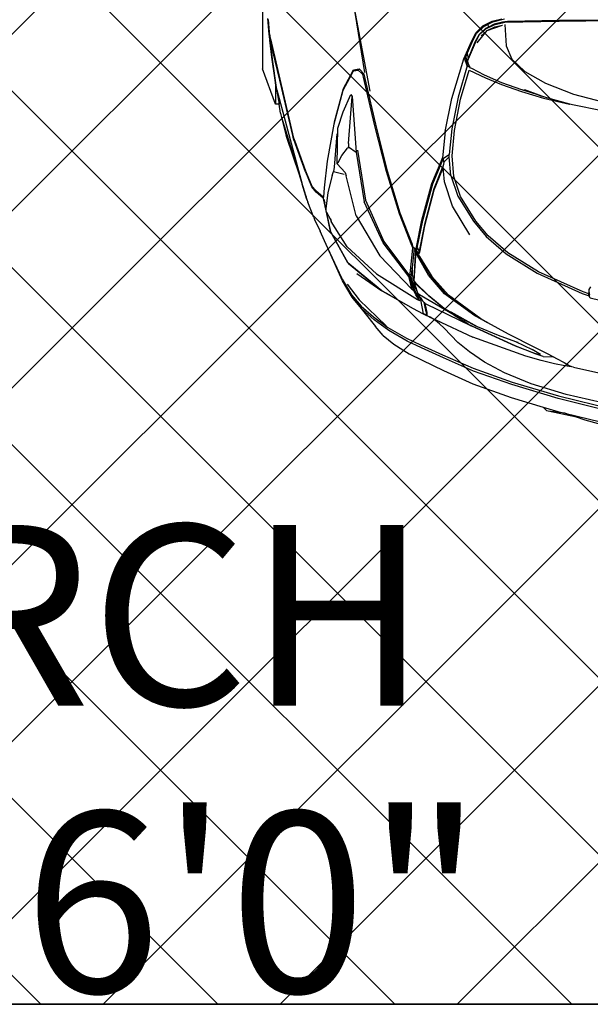
# Model space of a CAD drawing. Units: inches. Extents: x 2167 to 2589, y 1680 to 2489.
# Tile 12 of 38: x 2335 to 2358, y 1688 to 1727. Entities that reach past the tile are written whole.
import ezdxf

# ---------------------------------------------------------------- set-up
doc = ezdxf.new("R2010")
doc.units = ezdxf.units.IN
doc.header["$MEASUREMENT"] = 0
doc.layers.get('0').update_dxf_attribs({"color": 250})
for name, color, linetype, lineweight in [('A-AREA-IDEN', 7, 'Continuous', 18), ('C-PRKG-VEHS', 8, 'Continuous', 13), ('C-PROP', 7, 'Continuous', 35), ('L-PVMT-PATT', 252, 'Continuous', 13)]:
    doc.layers.add(name, color=color, linetype=linetype, lineweight=lineweight)
doc.layers.add('Edges', color=250, linetype='Continuous')
doc.styles.get("Standard").update_dxf_attribs({"font": 'arial.ttf'})

# ---------------------------------------------------------------- blocks, each defined once
blk = doc.blocks.new('Nissan Qashqai pl')
at = {"layer": 'Edges'}
for p, q in [((11.0595, 11.5599), (11.0607, 11.4508)), ((11.0606, 11.5601), (11.0618, 11.4509)), ((11.164, 11.4711), (11.1776, 11.5231)), ((11.6016, 11.5276), (11.5866, 11.4607)), ((11.5884, 11.4499), (11.6076, 11.5276)), ((11.6118, 11.5276), (11.5922, 11.4494)), ((11.6127, 11.4589), (11.6297, 11.5276)), ((11.1877, 11.5111), (11.1791, 11.4696)), ((11.4503, 11.4945), (11.4568, 11.5197)), ((11.5481, 11.471), (11.5571, 11.511)), ((11.435, 11.4947), (11.439, 11.4927)), ((11.439, 11.4927), (11.4437, 11.4925)), ((11.4451, 11.4934), (11.4432, 11.4935)), ((11.4437, 11.4925), (11.4449, 11.4929)), ((11.4445, 11.4833), (11.4478, 11.493)), ((11.4449, 11.4929), (11.4447, 11.4924)), ((11.4449, 11.4929), (11.4461, 11.4934)), ((11.4451, 11.4934), (11.4449, 11.4929)), ((11.4461, 11.4934), (11.4451, 11.4934)), ((11.4479, 11.4933), (11.4461, 11.4934)), ((11.4479, 11.4933), (11.4462, 11.4924)), ((11.4478, 11.493), (11.4462, 11.4924)), ((11.4502, 11.4939), (11.4478, 11.493)), ((11.4503, 11.4945), (11.4479, 11.4932)), ((11.4479, 11.4932), (11.4479, 11.4933)), ((11.4502, 11.4939), (11.4503, 11.4945)), ((11.6277, 11.5063), (11.6224, 11.4874)), ((11.4422, 11.4848), (11.4138, 11.4219)), ((11.4159, 11.42), (11.4445, 11.4833)), ((11.4447, 11.4924), (11.4422, 11.4848)), ((11.4447, 11.4924), (11.4437, 11.4925)), ((11.4462, 11.4924), (11.4447, 11.4924)), ((11.6224, 11.4874), (11.6185, 11.4753)), ((11.1487, 11.4316), (11.164, 11.4711)), ((11.1781, 11.4659), (11.1694, 11.4337)), ((11.1699, 11.4289), (11.178, 11.4652)), ((11.178, 11.4652), (11.1781, 11.4659)), ((11.1791, 11.4696), (11.1781, 11.4659)), ((11.5455, 11.4648), (11.5472, 11.4684)), ((11.5481, 11.471), (11.5467, 11.462)), ((11.6185, 11.4753), (11.6101, 11.4356)), ((11.6174, 11.472), (11.6127, 11.4589)), ((11.6185, 11.4753), (11.6174, 11.472)), ((11.5357, 11.4473), (11.5416, 11.4578)), ((11.5416, 11.4578), (11.5455, 11.4648)), ((11.5461, 11.4587), (11.5434, 11.4445)), ((11.5467, 11.462), (11.5461, 11.4587)), ((11.5866, 11.4607), (11.5715, 11.4115)), ((11.6127, 11.4589), (11.6101, 11.4356)), ((11.6103, 11.4492), (11.6127, 11.4589)), ((11.0607, 11.4508), (11.0621, 11.3784)), ((11.0618, 11.4509), (11.0632, 11.3741)), ((11.5283, 11.4332), (11.5334, 11.4428)), ((11.5326, 11.4397), (11.5333, 11.4423)), ((11.5331, 11.4285), (11.5335, 11.4431)), ((11.5333, 11.4423), (11.5334, 11.4428)), ((11.5334, 11.4428), (11.5335, 11.4431)), ((11.5335, 11.4431), (11.5357, 11.4473)), ((11.5434, 11.4445), (11.5386, 11.4254)), ((11.5691, 11.385), (11.5884, 11.4499)), ((11.5922, 11.4494), (11.5726, 11.3842)), ((11.6042, 11.4286), (11.6103, 11.4492)), ((11.1323, 11.4027), (11.1487, 11.4316)), ((11.1668, 11.4265), (11.1582, 11.4026)), ((11.1605, 11.3977), (11.1699, 11.4289)), ((11.1643, 11.4192), (11.1668, 11.4265)), ((11.1694, 11.4337), (11.1668, 11.4265)), ((11.5202, 11.4171), (11.5283, 11.4332)), ((11.5301, 11.4244), (11.523, 11.4131)), ((11.5331, 11.4285), (11.5292, 11.417)), ((11.5302, 11.4232), (11.5301, 11.4244)), ((11.5386, 11.4254), (11.5325, 11.4038)), ((11.5908, 11.3836), (11.6042, 11.4286)), ((11.6077, 11.4316), (11.6042, 11.4286)), ((11.6094, 11.4335), (11.6077, 11.4316)), ((11.6101, 11.4356), (11.6094, 11.4335)), ((11.1576, 11.3983), (11.1643, 11.4192)), ((11.1577, 11.3977), (11.1643, 11.4192)), ((11.1643, 11.4192), (11.1583, 11.4019)), ((11.4138, 11.4219), (11.3872, 11.3788)), ((11.3888, 11.3764), (11.4159, 11.42)), ((11.5013, 11.3791), (11.5202, 11.4171)), ((11.5118, 11.3894), (11.523, 11.4131)), ((11.5292, 11.417), (11.5179, 11.389)), ((11.5179, 11.389), (11.5285, 11.4163)), ((11.5285, 11.4163), (11.5302, 11.4232)), ((11.5715, 11.4115), (11.5562, 11.3741)), ((11.1148, 11.3843), (11.1323, 11.4027)), ((11.1475, 11.37), (11.1577, 11.3977)), ((11.1505, 11.37), (11.1605, 11.3977)), ((11.5325, 11.4038), (11.5057, 11.3296)), ((11.0962, 11.3766), (11.1148, 11.3843)), ((11.5179, 11.389), (11.488, 11.3234)), ((11.49, 11.3275), (11.5179, 11.389)), ((11.5028, 11.365), (11.5118, 11.3894)), ((11.5118, 11.3894), (11.513, 11.3927)), ((11.5496, 11.33), (11.5691, 11.385)), ((11.5726, 11.3842), (11.5535, 11.3303)), ((11.5716, 11.3297), (11.5908, 11.3836)), ((11.0614, 11.3569), (11.0581, 11.3704)), ((11.0624, 11.3576), (11.0582, 11.3742)), ((11.0621, 11.3784), (11.0622, 11.3745)), ((11.0622, 11.3745), (11.063, 11.3714)), ((11.063, 11.3714), (11.0659, 11.3594)), ((11.0632, 11.3741), (11.0641, 11.3708)), ((11.0641, 11.3708), (11.0669, 11.3592)), ((11.0662, 11.3744), (11.0962, 11.3766)), ((11.0696, 11.3606), (11.0671, 11.3711)), ((11.0747, 11.3498), (11.0671, 11.3711)), ((11.1369, 11.3455), (11.1475, 11.37)), ((11.1412, 11.3473), (11.1505, 11.37)), ((11.3872, 11.3788), (11.3635, 11.3513)), ((11.3645, 11.3484), (11.3888, 11.3764)), ((11.4852, 11.3502), (11.5013, 11.3791)), ((11.5562, 11.3741), (11.541, 11.3459)), ((11.0682, 11.3438), (11.0614, 11.3569)), ((11.0658, 11.3509), (11.0624, 11.3576)), ((11.0659, 11.3594), (11.0698, 11.3516)), ((11.0669, 11.3592), (11.0727, 11.3475)), ((11.0747, 11.3498), (11.0696, 11.3606)), ((11.4909, 11.3357), (11.5028, 11.365)), ((11.0698, 11.3516), (11.0658, 11.3509)), ((11.0692, 11.3445), (11.0658, 11.3509)), ((11.0779, 11.3339), (11.0682, 11.3438)), ((11.0787, 11.3349), (11.0692, 11.3445)), ((11.0698, 11.3516), (11.0718, 11.3475)), ((11.0718, 11.3475), (11.0802, 11.3384)), ((11.0727, 11.3475), (11.0809, 11.3386)), ((11.0821, 11.3412), (11.0747, 11.3498)), ((11.092, 11.3355), (11.0747, 11.3498)), ((11.1277, 11.3275), (11.1369, 11.3455)), ((11.1302, 11.3242), (11.1412, 11.3473)), ((11.3635, 11.3513), (11.3425, 11.3336)), ((11.3428, 11.3303), (11.3645, 11.3484)), ((11.48, 11.341), (11.4467, 11.2954)), ((11.4852, 11.3502), (11.4758, 11.3323)), ((11.4788, 11.339), (11.48, 11.341)), ((11.48, 11.341), (11.4801, 11.3411)), ((11.4801, 11.3411), (11.4852, 11.3502)), ((11.541, 11.3459), (11.5265, 11.3247)), ((11.0902, 11.3275), (11.0779, 11.3339)), ((11.0908, 11.3288), (11.0787, 11.3349)), ((11.0802, 11.3384), (11.0912, 11.3325)), ((11.0809, 11.3386), (11.0917, 11.3327)), ((11.1144, 11.3171), (11.0902, 11.3275)), ((11.107, 11.3218), (11.0908, 11.3288)), ((11.0912, 11.3325), (11.1138, 11.3229)), ((11.0917, 11.3327), (11.1149, 11.323)), ((11.1264, 11.325), (11.1277, 11.3275)), ((11.3076, 11.3083), (11.3428, 11.3303)), ((11.3425, 11.3336), (11.3082, 11.3121)), ((11.4433, 11.2899), (11.4745, 11.3325)), ((11.4758, 11.3323), (11.4447, 11.2897)), ((11.4633, 11.2847), (11.4897, 11.3334)), ((11.4704, 11.2984), (11.4909, 11.3357)), ((11.4704, 11.2984), (11.4897, 11.3334)), ((11.4788, 11.339), (11.4745, 11.3325)), ((11.4813, 11.2773), (11.5057, 11.3296)), ((11.4898, 11.3269), (11.4895, 11.3264)), ((11.4897, 11.3334), (11.4909, 11.3357)), ((11.4898, 11.3269), (11.49, 11.3275)), ((11.5306, 11.2869), (11.5496, 11.33)), ((11.5535, 11.3303), (11.5349, 11.2883)), ((11.5527, 11.2882), (11.5716, 11.3297)), ((11.107, 11.3218), (11.1138, 11.3229)), ((11.1116, 11.3198), (11.107, 11.3218)), ((11.1116, 11.3198), (11.1244, 11.3215)), ((11.1147, 11.3185), (11.1116, 11.3198)), ((11.1138, 11.3229), (11.1139, 11.3228)), ((11.1139, 11.3228), (11.1164, 11.3217)), ((11.1702, 11.2998), (11.1144, 11.3171)), ((11.1244, 11.3215), (11.1147, 11.3185)), ((11.1149, 11.323), (11.1172, 11.322)), ((11.1164, 11.3217), (11.1172, 11.322)), ((11.1174, 11.3219), (11.1164, 11.3217)), ((11.1172, 11.322), (11.1174, 11.3219)), ((11.1174, 11.3219), (11.12, 11.3227)), ((11.12, 11.3227), (11.1246, 11.3243)), ((11.126, 11.3248), (11.1244, 11.3215)), ((11.1244, 11.3215), (11.1259, 11.3248)), ((11.1244, 11.3215), (11.1684, 11.3087)), ((11.1246, 11.3243), (11.1259, 11.3248)), ((11.1247, 11.3244), (11.126, 11.3249)), ((11.1248, 11.3247), (11.126, 11.3249)), ((11.126, 11.3249), (11.1251, 11.3253)), ((11.1259, 11.3248), (11.126, 11.3249)), ((11.1259, 11.3248), (11.126, 11.3248)), ((11.126, 11.3249), (11.1263, 11.3255)), ((11.126, 11.3248), (11.1264, 11.325)), ((11.126, 11.3249), (11.1261, 11.3249)), ((11.1261, 11.3249), (11.126, 11.3248)), ((11.1263, 11.3254), (11.1261, 11.3249)), ((11.1261, 11.3249), (11.1264, 11.325)), ((11.1712, 11.3124), (11.1302, 11.3242)), ((11.3619, 11.3254), (11.3218, 11.3008)), ((11.4588, 11.2635), (11.4895, 11.3264)), ((11.475, 11.3032), (11.4828, 11.3165)), ((11.488, 11.3234), (11.4828, 11.3165)), ((11.5265, 11.3247), (11.5131, 11.3085)), ((11.1684, 11.3087), (11.2127, 11.2998)), ((11.2166, 11.2908), (11.1702, 11.2998)), ((11.2152, 11.3038), (11.1712, 11.3124)), ((11.2127, 11.2998), (11.2488, 11.2962)), ((11.2509, 11.3003), (11.2152, 11.3038)), ((11.28, 11.3028), (11.2509, 11.3003)), ((11.2785, 11.2987), (11.3076, 11.3083)), ((11.3082, 11.3121), (11.28, 11.3028)), ((11.3218, 11.3008), (11.2874, 11.2897)), ((11.475, 11.3032), (11.4462, 11.2548)), ((11.5131, 11.3085), (11.4933, 11.2891)), ((11.2166, 11.2908), (11.2538, 11.2871)), ((11.2524, 11.2965), (11.2488, 11.2962)), ((11.2541, 11.2885), (11.2488, 11.2962)), ((11.2785, 11.2987), (11.2524, 11.2965)), ((11.2524, 11.2965), (11.2599, 11.2889)), ((11.2586, 11.285), (11.2538, 11.2871)), ((11.2599, 11.2889), (11.2541, 11.2885)), ((11.29, 11.2731), (11.2541, 11.2885)), ((11.2895, 11.2718), (11.2586, 11.285)), ((11.2599, 11.2889), (11.26, 11.2889)), ((11.26, 11.2889), (11.265, 11.2879)), ((11.26, 11.2889), (11.2677, 11.2867)), ((11.2724, 11.2885), (11.265, 11.2879)), ((11.265, 11.2879), (11.2705, 11.2862)), ((11.2677, 11.2867), (11.2678, 11.2866)), ((11.2678, 11.2866), (11.2972, 11.2749)), ((11.2705, 11.2862), (11.2993, 11.2747)), ((11.2874, 11.2897), (11.2724, 11.2885)), ((11.4171, 11.2676), (11.4433, 11.2899)), ((11.4447, 11.2897), (11.4187, 11.2673)), ((11.4203, 11.2717), (11.4467, 11.2954)), ((11.4469, 11.2668), (11.4659, 11.2902)), ((11.4654, 11.2893), (11.4479, 11.2676)), ((11.4654, 11.2893), (11.4659, 11.2902)), ((11.4659, 11.2902), (11.4674, 11.2929)), ((11.4675, 11.2931), (11.4674, 11.2929)), ((11.4675, 11.2931), (11.4703, 11.2982)), ((11.4703, 11.2982), (11.4704, 11.2984)), ((11.4933, 11.2891), (11.4869, 11.2826)), ((11.5165, 11.256), (11.5306, 11.2869)), ((11.5349, 11.2883), (11.5206, 11.2572)), ((11.5384, 11.2583), (11.5527, 11.2882)), ((11.3411, 11.2579), (11.2895, 11.2718)), ((11.3419, 11.2592), (11.29, 11.2731)), ((11.2972, 11.2749), (11.3474, 11.2614)), ((11.2993, 11.2747), (11.3493, 11.2614)), ((11.3923, 11.2547), (11.4203, 11.2717)), ((11.4771, 11.2681), (11.4813, 11.2773)), ((11.4826, 11.2772), (11.4778, 11.2695)), ((11.4813, 11.2773), (11.4822, 11.2786)), ((11.4869, 11.2826), (11.4826, 11.2772)), ((11.3795, 11.2503), (11.3411, 11.2579)), ((11.3804, 11.2515), (11.3419, 11.2592)), ((11.3474, 11.2614), (11.3848, 11.2543)), ((11.3493, 11.2614), (11.3863, 11.2544)), ((11.4171, 11.2676), (11.3851, 11.2491)), ((11.4187, 11.2673), (11.3914, 11.2516)), ((11.4296, 11.2488), (11.4469, 11.2668)), ((11.4479, 11.2676), (11.4303, 11.2485)), ((11.4498, 11.2553), (11.4549, 11.2587)), ((11.4728, 11.2604), (11.4535, 11.2565)), ((11.4549, 11.2587), (11.4568, 11.2605)), ((11.4564, 11.2609), (11.4567, 11.2609)), ((11.4565, 11.261), (11.4569, 11.2611)), ((11.4568, 11.2605), (11.4571, 11.2609)), ((11.4571, 11.2609), (11.4573, 11.2612)), ((11.4704, 11.2639), (11.4573, 11.2612)), ((11.4573, 11.2612), (11.4578, 11.262)), ((11.4574, 11.2619), (11.4573, 11.2619)), ((11.4573, 11.2619), (11.4573, 11.2619)), ((11.4574, 11.2619), (11.4576, 11.2619)), ((11.4578, 11.262), (11.4588, 11.2635)), ((11.4578, 11.262), (11.4605, 11.2625)), ((11.4605, 11.2625), (11.4713, 11.2647)), ((11.4605, 11.2625), (11.4605, 11.2625)), ((11.4732, 11.2592), (11.4658, 11.2461)), ((11.4704, 11.2639), (11.4742, 11.2645)), ((11.4713, 11.2647), (11.4744, 11.265)), ((11.4727, 11.2601), (11.4728, 11.2603)), ((11.4746, 11.2646), (11.4728, 11.2604)), ((11.4742, 11.2645), (11.4728, 11.2604)), ((11.4728, 11.2603), (11.4732, 11.261)), ((11.4728, 11.2604), (11.4728, 11.2603)), ((11.4728, 11.2603), (11.4732, 11.2592)), ((11.4758, 11.2651), (11.4732, 11.2592)), ((11.4742, 11.2645), (11.4745, 11.2645)), ((11.4744, 11.265), (11.4743, 11.2647)), ((11.4744, 11.265), (11.4745, 11.265)), ((11.4745, 11.2648), (11.4745, 11.265)), ((11.4745, 11.265), (11.4748, 11.265)), ((11.4746, 11.2646), (11.4745, 11.2645)), ((11.4758, 11.2651), (11.4746, 11.2646)), ((11.4748, 11.265), (11.4747, 11.2648)), ((11.4748, 11.265), (11.4758, 11.2651)), ((11.4759, 11.2652), (11.4758, 11.2651)), ((11.4778, 11.2695), (11.4759, 11.2652)), ((11.4771, 11.2681), (11.4759, 11.2652)), ((11.5206, 11.2572), (11.5113, 11.2372)), ((11.5295, 11.24), (11.5384, 11.2583)), ((11.3311, 11.227), (11.3751, 11.2443)), ((11.38, 11.2453), (11.3747, 11.2431)), ((11.3751, 11.2443), (11.3752, 11.2444)), ((11.3751, 11.2443), (11.3762, 11.2443)), ((11.3792, 11.2459), (11.3752, 11.2444)), ((11.3763, 11.2444), (11.3752, 11.2444)), ((11.3792, 11.2459), (11.3804, 11.2469)), ((11.3793, 11.2463), (11.3792, 11.2459)), ((11.3834, 11.2495), (11.3795, 11.2503)), ((11.3853, 11.2449), (11.38, 11.2453)), ((11.3804, 11.2515), (11.3848, 11.2543)), ((11.3841, 11.2508), (11.3804, 11.2515)), ((11.3804, 11.2469), (11.3827, 11.2489)), ((11.3804, 11.2469), (11.4082, 11.2444)), ((11.3813, 11.2485), (11.3817, 11.2488)), ((11.3827, 11.2489), (11.3834, 11.2495)), ((11.3829, 11.249), (11.388, 11.2532)), ((11.3845, 11.2498), (11.3829, 11.249)), ((11.3829, 11.249), (11.3849, 11.2491)), ((11.3829, 11.249), (11.3846, 11.2488)), ((11.3841, 11.2508), (11.3834, 11.2495)), ((11.3846, 11.2489), (11.385, 11.2491)), ((11.3849, 11.2491), (11.3846, 11.2489)), ((11.3846, 11.2488), (11.3846, 11.2489)), ((11.3846, 11.2488), (11.3893, 11.2486)), ((11.3848, 11.2543), (11.388, 11.2532)), ((11.3882, 11.2519), (11.3849, 11.2491)), ((11.385, 11.2491), (11.3851, 11.2491)), ((11.3851, 11.2491), (11.3867, 11.2492)), ((11.4212, 11.2412), (11.3853, 11.2449)), ((11.3881, 11.2519), (11.3861, 11.2508)), ((11.3863, 11.2544), (11.3895, 11.253)), ((11.3914, 11.2516), (11.3867, 11.2492)), ((11.3867, 11.2492), (11.3915, 11.2491)), ((11.3886, 11.2522), (11.3882, 11.2519)), ((11.3886, 11.2522), (11.3882, 11.252)), ((11.3906, 11.2534), (11.3886, 11.2522)), ((11.3895, 11.253), (11.3886, 11.2522)), ((11.3893, 11.2486), (11.4248, 11.2465)), ((11.3895, 11.253), (11.3923, 11.2547)), ((11.3915, 11.2491), (11.4266, 11.2465)), ((11.3915, 11.1988), (11.4381, 11.244)), ((11.4164, 11.2444), (11.4082, 11.2444)), ((11.409, 11.2443), (11.4082, 11.2444)), ((11.409, 11.2443), (11.4163, 11.2443)), ((11.4152, 11.2437), (11.409, 11.2443)), ((11.4163, 11.2443), (11.4152, 11.2437)), ((11.4215, 11.2431), (11.4152, 11.2437)), ((11.4164, 11.2444), (11.4163, 11.2443)), ((11.4169, 11.2446), (11.4164, 11.2444)), ((11.4252, 11.2462), (11.4169, 11.2446)), ((11.417, 11.1942), (11.4529, 11.252)), ((11.423, 11.2435), (11.4215, 11.2431)), ((11.4315, 11.244), (11.4229, 11.2416)), ((11.423, 11.2435), (11.4229, 11.2416)), ((11.44, 11.2482), (11.423, 11.2435)), ((11.4248, 11.2465), (11.4266, 11.2465)), ((11.4266, 11.2465), (11.4252, 11.2462)), ((11.4266, 11.2465), (11.4268, 11.2465)), ((11.4268, 11.2465), (11.4296, 11.2488)), ((11.4268, 11.2465), (11.4278, 11.2465)), ((11.4303, 11.2485), (11.4278, 11.2465)), ((11.4278, 11.2465), (11.43, 11.2472)), ((11.4381, 11.244), (11.4292, 11.2418)), ((11.43, 11.2472), (11.4361, 11.2494)), ((11.4337, 11.248), (11.43, 11.2472)), ((11.4403, 11.2464), (11.4315, 11.244)), ((11.4397, 11.2505), (11.4337, 11.248)), ((11.4361, 11.2494), (11.4406, 11.251)), ((11.4381, 11.244), (11.4403, 11.2464)), ((11.4406, 11.251), (11.4397, 11.2505)), ((11.4457, 11.2513), (11.44, 11.2482)), ((11.4403, 11.2464), (11.44, 11.2482)), ((11.4462, 11.2495), (11.4403, 11.2464)), ((11.4406, 11.251), (11.4442, 11.2522)), ((11.4411, 11.2028), (11.4656, 11.2458)), ((11.4442, 11.2522), (11.4497, 11.2552)), ((11.4462, 11.2548), (11.4442, 11.2522)), ((11.4512, 11.2549), (11.4457, 11.2513)), ((11.452, 11.2532), (11.4462, 11.2495)), ((11.447, 11.2127), (11.4656, 11.2458)), ((11.4497, 11.2552), (11.4498, 11.2553)), ((11.4498, 11.2553), (11.4535, 11.2565)), ((11.4512, 11.2549), (11.4535, 11.2565)), ((11.4539, 11.2545), (11.452, 11.2532)), ((11.4529, 11.252), (11.4542, 11.2547)), ((11.4532, 11.256), (11.4535, 11.2565)), ((11.4535, 11.2565), (11.4542, 11.2547)), ((11.4542, 11.2547), (11.4539, 11.2545)), ((11.4656, 11.2458), (11.4658, 11.2461)), ((11.472, 11.2571), (11.4718, 11.2568)), ((11.5074, 11.2362), (11.5165, 11.256)), ((11.3747, 11.2431), (11.3323, 11.2264)), ((11.3715, 11.2043), (11.4177, 11.2389)), ((11.4203, 11.2398), (11.3733, 11.2037)), ((11.4177, 11.2389), (11.4193, 11.24)), ((11.4192, 11.2397), (11.4194, 11.24)), ((11.4193, 11.24), (11.4196, 11.2402)), ((11.4194, 11.24), (11.4193, 11.24)), ((11.4194, 11.24), (11.4196, 11.2402)), ((11.4196, 11.2399), (11.4194, 11.24)), ((11.4196, 11.2402), (11.4201, 11.2405)), ((11.4198, 11.2401), (11.4201, 11.2405)), ((11.4201, 11.2405), (11.4212, 11.2412)), ((11.4292, 11.2418), (11.4203, 11.2398)), ((11.4229, 11.2416), (11.4203, 11.2398)), ((11.4212, 11.2412), (11.4215, 11.2431)), ((11.4218, 11.2413), (11.4212, 11.2412)), ((11.4229, 11.2416), (11.4218, 11.2413)), ((11.4222, 11.2413), (11.4218, 11.2413)), ((11.4924, 11.2103), (11.5074, 11.2362)), ((11.5113, 11.2372), (11.4963, 11.2114)), ((11.5158, 11.2186), (11.5295, 11.24)), ((11.272, 11.2092), (11.3311, 11.227)), ((11.3323, 11.2264), (11.2728, 11.2084)), ((11.5033, 11.2034), (11.5158, 11.2186)), ((11.2063, 11.1926), (11.272, 11.2092)), ((11.2728, 11.2084), (11.2066, 11.1914)), ((11.3132, 11.1789), (11.3715, 11.2043)), ((11.3733, 11.2037), (11.3153, 11.1769)), ((11.4405, 11.2018), (11.4014, 11.1541)), ((11.4022, 11.1548), (11.4405, 11.2018)), ((11.4163, 11.1666), (11.4405, 11.2018)), ((11.4408, 11.2022), (11.4405, 11.2018)), ((11.4411, 11.2028), (11.4408, 11.2022)), ((11.447, 11.2127), (11.4411, 11.2028)), ((11.4411, 11.2028), (11.4411, 11.2028)), ((11.4531, 11.1697), (11.4897, 11.2077)), ((11.4774, 11.1898), (11.4924, 11.2103)), ((11.4963, 11.2114), (11.4815, 11.191)), ((11.5033, 11.2034), (11.4936, 11.195)), ((11.2066, 11.1914), (11.1401, 11.1759)), ((11.148, 11.1791), (11.2063, 11.1926)), ((11.335, 11.1656), (11.3915, 11.1988)), ((11.379, 11.1527), (11.417, 11.1942)), ((11.4543, 11.1636), (11.4908, 11.1928)), ((11.4624, 11.1725), (11.4774, 11.1898)), ((11.4815, 11.191), (11.4662, 11.1736)), ((11.4936, 11.195), (11.4908, 11.1928)), ((11.0357, 11.1613), (11.1598, 11.1847)), ((11.0492, 11.1635), (11.1336, 11.1772)), ((11.1293, 11.1705), (11.1353, 11.1764)), ((11.1366, 11.175), (11.1347, 11.1731)), ((11.1353, 11.1764), (11.1358, 11.1765)), ((11.1358, 11.1765), (11.148, 11.1791)), ((11.1358, 11.1765), (11.1366, 11.175)), ((11.1401, 11.1759), (11.1366, 11.175)), ((11.2428, 11.1673), (11.3132, 11.1789)), ((11.2459, 11.1656), (11.3153, 11.1769)), ((11.1285, 11.1697), (11.1293, 11.1705)), ((11.1298, 11.1618), (11.1285, 11.1697)), ((11.1293, 11.1705), (11.1306, 11.163)), ((11.156, 11.1476), (11.1298, 11.1618)), ((11.1347, 11.1731), (11.1306, 11.169)), ((11.1306, 11.169), (11.1319, 11.1614)), ((11.1319, 11.1614), (11.1306, 11.163)), ((11.1319, 11.1614), (11.1365, 11.159)), ((11.1672, 11.1598), (11.2459, 11.1656)), ((11.2382, 11.1549), (11.2459, 11.1656)), ((11.335, 11.1656), (11.2791, 11.1515)), ((11.4314, 11.1531), (11.4531, 11.1697)), ((11.4464, 11.1588), (11.4624, 11.1725)), ((11.4543, 11.1636), (11.4498, 11.1598)), ((11.4662, 11.1736), (11.4543, 11.1636)), ((11.1365, 11.159), (11.1589, 11.147)), ((11.2029, 11.1349), (11.156, 11.1476)), ((11.1589, 11.147), (11.2062, 11.1344)), ((11.1644, 11.1579), (11.1672, 11.1598)), ((11.189, 11.1473), (11.1644, 11.1579)), ((11.2337, 11.155), (11.1672, 11.1598)), ((11.2121, 11.1399), (11.189, 11.1473)), ((11.2337, 11.155), (11.2382, 11.1549)), ((11.2382, 11.1549), (11.2401, 11.1534)), ((11.2505, 11.1455), (11.2401, 11.1534)), ((11.2743, 11.1499), (11.2622, 11.139)), ((11.2729, 11.1338), (11.2766, 11.1485)), ((11.2743, 11.1499), (11.2791, 11.1515)), ((11.379, 11.1527), (11.3434, 11.1303)), ((11.4014, 11.1541), (11.3571, 11.1296)), ((11.3583, 11.13), (11.4014, 11.1541)), ((11.4022, 11.1548), (11.4014, 11.1541)), ((11.4243, 11.1459), (11.4464, 11.1588)), ((11.4498, 11.1598), (11.4267, 11.1463)), ((11.2029, 11.1349), (11.2029, 11.1349)), ((11.2029, 11.1349), (11.2062, 11.1344)), ((11.2062, 11.1344), (11.2583, 11.1246)), ((11.2622, 11.139), (11.2121, 11.1399)), ((11.2199, 11.1382), (11.2666, 11.1345)), ((11.2601, 11.1405), (11.2505, 11.1455)), ((11.2622, 11.139), (11.2601, 11.1405)), ((11.2666, 11.1345), (11.2729, 11.1338)), ((11.2787, 11.1318), (11.2729, 11.1338)), ((11.4267, 11.1463), (11.3807, 11.1259)), ((11.4228, 11.1453), (11.3807, 11.1259)), ((11.4228, 11.1453), (11.4243, 11.1459)), ((11.2583, 11.1246), (11.2956, 11.1208)), ((11.2787, 11.1318), (11.3022, 11.1256)), ((11.2956, 11.1208), (11.3085, 11.1195)), ((11.3, 11.1092), (11.3081, 11.1188)), ((11.3103, 11.1192), (11.3018, 11.1096)), ((11.3022, 11.1256), (11.3252, 11.1229)), ((11.308, 11.1188), (11.3086, 11.1195)), ((11.3081, 11.1188), (11.3086, 11.1195)), ((11.3085, 11.1195), (11.3086, 11.1195)), ((11.3086, 11.1195), (11.3103, 11.1193)), ((11.3103, 11.1193), (11.3103, 11.1192)), ((11.3103, 11.1193), (11.3106, 11.1193)), ((11.3106, 11.1193), (11.314, 11.1204)), ((11.317, 11.1214), (11.3119, 11.1206)), ((11.3132, 11.1199), (11.3259, 11.1227)), ((11.3242, 11.1226), (11.314, 11.1204)), ((11.314, 11.1204), (11.317, 11.1214)), ((11.3242, 11.1226), (11.317, 11.1214)), ((11.3198, 11.1231), (11.3252, 11.1229)), ((11.3242, 11.1226), (11.3259, 11.1227)), ((11.3252, 11.1229), (11.3283, 11.1228)), ((11.3259, 11.1227), (11.3283, 11.1228)), ((11.3283, 11.1228), (11.3296, 11.1235)), ((11.3296, 11.1235), (11.3571, 11.1296)), ((11.3296, 11.1235), (11.3302, 11.1238)), ((11.3571, 11.1296), (11.3302, 11.1238)), ((11.3302, 11.1238), (11.3394, 11.129)), ((11.3394, 11.129), (11.342, 11.1305)), ((11.3394, 11.129), (11.3434, 11.1303)), ((11.3796, 11.1255), (11.3566, 11.1148)), ((11.3571, 11.1296), (11.3583, 11.13)), ((11.3807, 11.1259), (11.3796, 11.1255)), ((11.2934, 11.1031), (11.3, 11.1092)), ((11.3018, 11.1096), (11.2946, 11.1033)), ((11.3376, 11.106), (11.3161, 11.0975)), ((11.3376, 11.106), (11.3405, 11.1072)), ((11.3405, 11.1072), (11.3566, 11.1148)), ((11.2732, 11.0945), (11.2277, 11.0779)), ((11.2304, 11.0792), (11.2719, 11.0943)), ((11.2719, 11.0943), (11.2741, 11.0952)), ((11.2736, 11.0947), (11.2732, 11.0945)), ((11.2946, 11.1033), (11.2736, 11.0947)), ((11.2736, 11.0947), (11.2741, 11.0952)), ((11.2741, 11.0952), (11.2934, 11.1031)), ((11.2757, 11.085), (11.3124, 11.0963)), ((11.3124, 11.0963), (11.2907, 11.0899)), ((11.308, 11.0951), (11.3088, 11.0953)), ((11.3124, 11.0963), (11.3161, 11.0975)), ((11.1582, 11.0542), (11.2907, 11.0899)), ((11.1963, 11.0607), (11.2757, 11.085)), ((11.2271, 11.0777), (11.2222, 11.0766)), ((11.2224, 11.0767), (11.2253, 11.0774)), ((11.2247, 11.0677), (11.2757, 11.085)), ((11.2253, 11.0774), (11.2304, 11.0792)), ((11.2296, 11.0784), (11.2271, 11.0777)), ((11.2277, 11.0779), (11.2271, 11.0777)), ((11.2273, 11.0778), (11.2271, 11.0778)), ((11.2296, 11.0784), (11.2277, 11.0779)), ((11.0865, 11.045), (11.22, 11.0761)), ((11.2222, 11.0766), (11.0882, 11.045)), ((11.0918, 11.0453), (11.2222, 11.0766)), ((11.193, 11.0596), (11.2215, 11.0666)), ((11.22, 11.0761), (11.2222, 11.0766)), ((11.2215, 11.0666), (11.2247, 11.0677)), ((11.2224, 11.0767), (11.2222, 11.0766)), ((11.2222, 11.0766), (11.2222, 11.0766)), ((11.1475, 11.0521), (11.1123, 11.0472)), ((11.1147, 11.0476), (11.1547, 11.0532)), ((11.1783, 11.0521), (11.1283, 11.0341)), ((11.1525, 11.0528), (11.1475, 11.0521)), ((11.1475, 11.0521), (11.1783, 11.0521)), ((11.1547, 11.0532), (11.1525, 11.0528)), ((11.1547, 11.0532), (11.1783, 11.0572)), ((11.1906, 11.0592), (11.1783, 11.0572)), ((11.1783, 11.0572), (11.1783, 11.0521)), ((11.1909, 11.0593), (11.1906, 11.0592)), ((11.1909, 11.0593), (11.193, 11.0596)), ((11.0798, 11.0434), (11.0576, 11.0416)), ((11.059, 11.0419), (11.0768, 11.0434)), ((11.0768, 11.0434), (11.0811, 11.0437)), ((11.087, 11.0442), (11.0798, 11.0434)), ((11.0811, 11.0444), (11.0821, 11.0442)), ((11.0811, 11.0437), (11.0827, 11.0441)), ((11.0827, 11.0441), (11.0856, 11.0448)), ((11.0827, 11.0441), (11.0836, 11.0439)), ((11.0882, 11.045), (11.0836, 11.0439)), ((11.0836, 11.0439), (11.087, 11.0442)), ((11.0856, 11.0448), (11.0865, 11.045)), ((11.0865, 11.045), (11.088, 11.0451)), ((11.087, 11.0442), (11.0872, 11.0442)), ((11.0873, 11.0443), (11.0872, 11.0442)), ((11.0873, 11.0443), (11.0883, 11.0444)), ((11.0883, 11.0444), (11.1147, 11.0476)), ((11.1123, 11.0472), (11.0883, 11.0444)), ((10.9577, 11.0341), (11.1283, 11.0341))]:
    blk.add_line(p, q, dxfattribs=at)
blk = doc.blocks.new('car')
blk.add_blockref('Nissan Qashqai pl', (-9.7433, -11.9151))
blk = doc.blocks.new('carr')
blk.add_blockref('car', (0.5124, -0.007))

msp = doc.modelspace()

# ---------------------------------------------------------------- hatches: boundary and pattern name
at = {"layer": 'L-PVMT-PATT'}
h = msp.add_hatch(dxfattribs=at)
h.set_pattern_fill('ANSI37', color=256, scale=40)
h.paths.add_polyline_path([(2417.548, 1783.695), (2417.548, 1846.042), (2239.361, 1846.042), (2239.361, 1687.695), (2369.843, 1687.695), (2369.843, 1696.695), (2375.607, 1696.695), (2416.107, 1696.695), (2417.548, 1696.695)])

# ---------------------------------------------------------------- linework, layer by layer
at = {"layer": 'C-PROP'}
msp.add_line((2575.048, 1687.695), (2215.048, 1687.695), dxfattribs=at)

# ---------------------------------------------------------------- block references
at = {"layer": 'C-PRKG-VEHS', "xscale": 28.42784210623918, "yscale": 28.42784210623918, "zscale": 28.42784210623918, "rotation": 270}
msp.add_blockref('carr', (2369.852, 1779.037), dxfattribs=at)

# ---------------------------------------------------------------- texts
at = {"layer": 'A-AREA-IDEN'}
for s, height, p in [('CAR PORCH', 7.2272, (2297.172, 1699.634)), ('16\'0" X 16\'0"', 7.22716, (2295.694, 1688.165))]:
    msp.add_text(s, height=height, dxfattribs=at).set_placement(p)

doc.saveas('drawing.dxf')
